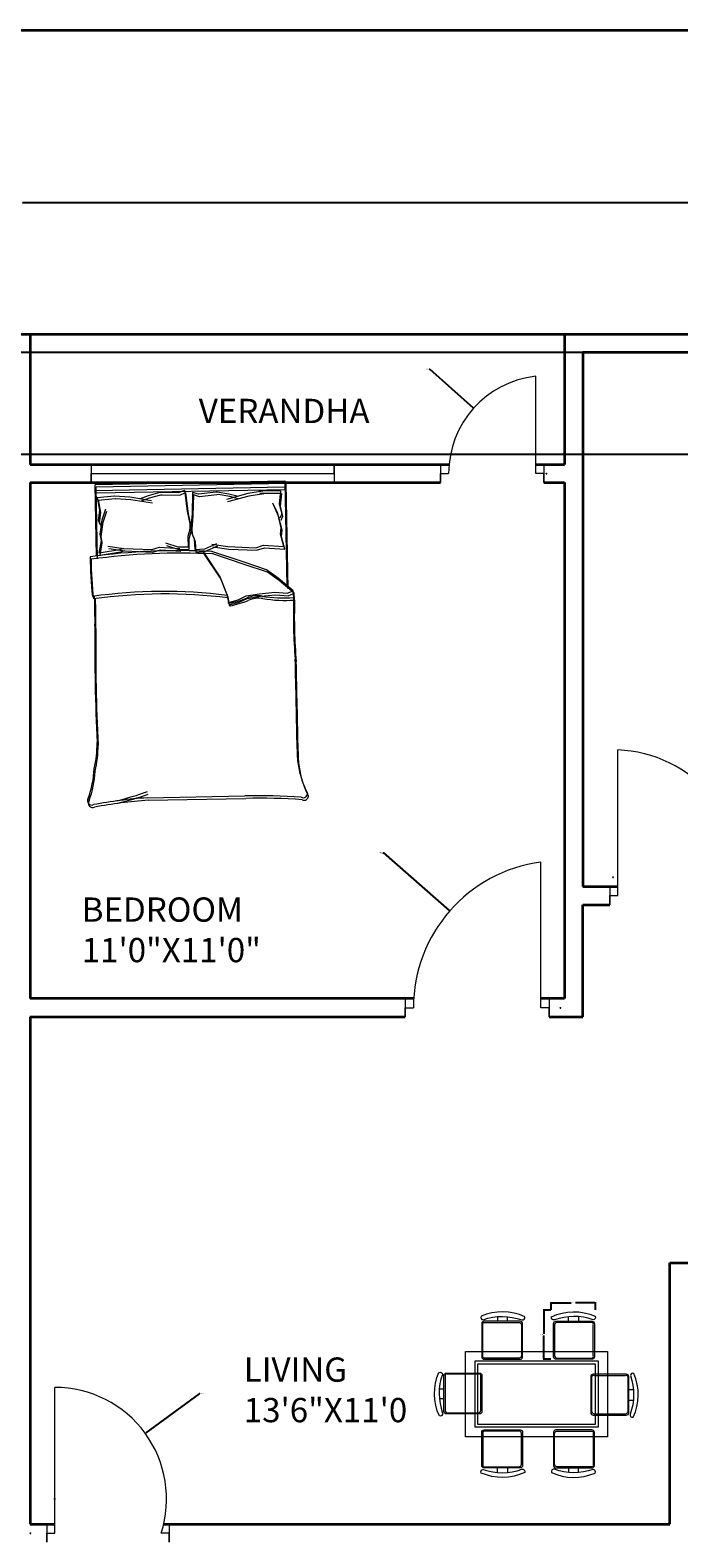
# Model space of a CAD drawing. Units: inches. Extents: x 1721 to 2510, y 1544 to 2360.
# Tile 9 of 10: x 2090 to 2250, y 1988 to 2360. Entities that reach past the tile are written whole.
import ezdxf

# ---------------------------------------------------------------- set-up
doc = ezdxf.new("R2010")
doc.units = ezdxf.units.IN
for name, color, linetype, lineweight in [('A-ANNO-DIMS', 2, 'Continuous', 18), ('A-ANNO-TTLB', 7, 'Continuous', 35), ('A-AREA-IDEN', 7, 'Continuous', 18), ('A-DOOR', 3, 'Continuous', 18), ('A-FURN', 8, 'Continuous', 13), ('A-GLAZ', 4, 'Continuous', 18), ('A-WALL', 7, 'Continuous', 35)]:
    doc.layers.add(name, color=color, linetype=linetype, lineweight=lineweight)
doc.styles.get("Standard").update_dxf_attribs({"font": 'arial.ttf'})
doc.dimstyles.get("Standard").update_dxf_attribs({"dimtxt": 0.18, "dimasz": 0.18, "dimexe": 0.18, "dimexo": 0.0625, "dimgap": 0.09, "dimtad": 0, "dimtih": 1, "dimtoh": 1, "dimdec": 4, "dimzin": 0, "dimdsep": 46, "dimtxsty": 'Standard', "dimcen": 0.09, "dimadec": 0, "dimazin": 0, "dimtfac": 1, "dimtdec": 4, "dimtofl": 0, "dimtmove": 0, "dimatfit": 3, "dimfxl": 1, "dimtolj": 1, "dimtzin": 0, "dimarcsym": 0})

# ---------------------------------------------------------------- blocks, each defined once
blk = doc.blocks.new('BED-DOUBLE')
for p, q in [((39.64, 78.43), (15.52, 78.72)), ((39.64, 78.43), (15.52, 78.72)), ((39.86, 77.8), (15.74, 78.09)), ((39.86, 77.8), (15.74, 78.09)), ((1.93, 30.11), (1.99, 28.4, 3.79)), ((1.93, 30.11), (1.99, 28.4, 3.79)), ((15.66, 30.21), (13.68, 29.32)), ((15.66, 30.21), (13.68, 29.32)), ((18.1, 30.79), (15.66, 30.21)), ((18.1, 30.79), (15.66, 30.21)), ((18.31, 30.16), (15.88, 29.58)), ((18.31, 30.16), (15.88, 29.58)), ((18.38, 28.81), (18.1, 30.79)), ((18.38, 28.81), (18.1, 30.79)), ((18.59, 28.18), (18.31, 30.16)), ((18.59, 28.18), (18.31, 30.16)), ((3.5, 28.99), (1.99, 28.4)), ((3.5, 28.99), (1.99, 28.4)), ((1.99, 28.4), (5.58, 25.17)), ((1.99, 28.4), (5.58, 25.17)), ((2.15, 29.48), (2.21, 27.77, 3.79)), ((2.15, 29.48), (2.21, 27.77, 3.79)), ((3.72, 28.36), (2.21, 27.77)), ((3.72, 28.36), (2.21, 27.77)), ((2.21, 27.77), (5.8, 24.54)), ((2.21, 27.77), (5.8, 24.54)), ((3.23, 1.19), (3.55, 27.27)), ((3.23, 1.19), (3.55, 27.27)), ((3.45, 0.56), (3.76, 26.64)), ((3.45, 0.56), (3.76, 26.64)), ((6.54, 28.65), (3.5, 28.99)), ((6.54, 28.65), (3.5, 28.99)), ((6.75, 28.02), (3.72, 28.36)), ((6.75, 28.02), (3.72, 28.36)), ((10.33, 28.91), (6.54, 28.65)), ((10.33, 28.91), (6.54, 28.65)), ((10.55, 28.28), (6.75, 28.02)), ((10.55, 28.28), (6.75, 28.02)), ((13.68, 29.32), (10.33, 28.91)), ((13.68, 29.32), (10.33, 28.91)), ((13.89, 28.69), (10.55, 28.28)), ((13.89, 28.69), (10.55, 28.28)), ((15.88, 29.58), (13.89, 28.69)), ((15.88, 29.58), (13.89, 28.69)), ((20, 24.39), (18.38, 28.81)), ((20, 24.39), (18.38, 28.81)), ((20.21, 23.76), (18.59, 28.18)), ((20.21, 23.76), (18.59, 28.18)), ((5.58, 25.17), (8.44, 23.01)), ((5.58, 25.17), (8.44, 23.01)), ((5.8, 24.54), (8.66, 22.38)), ((5.8, 24.54), (8.66, 22.38)), ((8.44, 23.01), (13.88, 20.98)), ((8.44, 23.01), (13.88, 20.98)), ((8.66, 22.38), (14.1, 20.35)), ((8.66, 22.38), (14.1, 20.35)), ((24.03, 17.98), (20, 24.39)), ((24.03, 17.98), (20, 24.39)), ((24.24, 17.35), (20.21, 23.76)), ((24.24, 17.35), (20.21, 23.76)), ((13.88, 20.98), (22.02, 18)), ((13.88, 20.98), (22.02, 18)), ((14.1, 20.35), (22.24, 17.37)), ((14.1, 20.35), (22.24, 17.37)), ((9.01, 16.97), (3.98, 17.42)), ((3.98, 17.42), (4.71, 14.34)), ((9.01, 16.97), (3.98, 17.42)), ((3.98, 17.42), (4.71, 14.34)), ((9.23, 16.34), (4.2, 16.8)), ((4.2, 16.8), (4.92, 13.71)), ((9.23, 16.34), (4.2, 16.8)), ((4.2, 16.8), (4.92, 13.71)), ((10.94, 17.49), (9.01, 16.97)), ((10.94, 17.49), (9.01, 16.97)), ((11.15, 16.86), (9.23, 16.34)), ((11.15, 16.86), (9.23, 16.34)), ((17.8, 16.99), (10.94, 17.49)), ((17.8, 16.99), (10.94, 17.49)), ((18.02, 16.36), (11.15, 16.86)), ((18.02, 16.36), (11.15, 16.86)), ((21.75, 16.29), (17.8, 16.99)), ((21.75, 16.29), (17.8, 16.99)), ((21.96, 15.66), (18.02, 16.36)), ((21.96, 15.66), (18.02, 16.36)), ((23.54, 17.35), (20.51, 16.13)), ((23.54, 17.35), (20.51, 16.13)), ((23.75, 16.73), (20.73, 15.5)), ((23.75, 16.73), (20.73, 15.5)), ((25.94, 17.48), (23.54, 17.35)), ((25.94, 17.48), (23.54, 17.35)), ((26.16, 16.85), (23.75, 16.73)), ((26.16, 16.85), (23.75, 16.73)), ((26.07, 14.85), (25.94, 17.48)), ((26.07, 14.85), (25.94, 17.48)), ((26.29, 14.22), (26.16, 16.85)), ((26.29, 14.22), (26.16, 16.85)), ((27.61, 14.21), (27.64, 16.84)), ((27.61, 14.21), (27.64, 16.84)), ((27.64, 16.84), (30.05, 16.81)), ((27.64, 16.84), (30.05, 16.81)), ((27.82, 13.58), (27.85, 16.21)), ((27.82, 13.58), (27.85, 16.21)), ((27.85, 16.21), (30.26, 16.18)), ((27.85, 16.21), (30.26, 16.18)), ((34.67, 16.66), (29.65, 17.12)), ((34.67, 16.66), (29.65, 17.12)), ((34.89, 16.03), (29.86, 16.49)), ((34.89, 16.03), (29.86, 16.49)), ((30.05, 16.81), (33.11, 15.7)), ((30.05, 16.81), (33.11, 15.7)), ((30.26, 16.18), (33.33, 15.07)), ((30.26, 16.18), (33.33, 15.07)), ((36.6, 17.19), (34.67, 16.66)), ((36.6, 17.19), (34.67, 16.66)), ((36.81, 16.56), (34.89, 16.03)), ((36.81, 16.56), (34.89, 16.03)), ((43.46, 16.68), (36.6, 17.19)), ((43.46, 16.68), (36.6, 17.19)), ((43.68, 16.05), (36.81, 16.56)), ((43.68, 16.05), (36.81, 16.56)), ((43.46, 16.68), (44.58, 16.98)), ((43.46, 16.68), (44.58, 16.98)), ((47.41, 15.98), (43.46, 16.68)), ((47.41, 15.98), (43.46, 16.68)), ((43.68, 16.05), (44.79, 16.35)), ((43.68, 16.05), (44.79, 16.35)), ((47.62, 15.35), (43.68, 16.05)), ((47.62, 15.35), (43.68, 16.05)), ((44.58, 16.98), (49.58, 17.63)), ((44.58, 16.98), (49.58, 17.63)), ((44.79, 16.35), (49.8, 17)), ((44.79, 16.35), (49.8, 17)), ((49.58, 17.63), (48.98, 14.52)), ((49.58, 17.63), (48.98, 14.52)), ((49.8, 17), (49.19, 13.89)), ((49.8, 17), (49.19, 13.89)), ((50.28, 18.38), (50.07, 0.63)), ((50.28, 18.38), (50.07, 0.63)), ((50.5, 17.75), (50.29, 0)), ((50.5, 17.75), (50.29, 0)), ((4.71, 14.34), (4.5, 12.77)), ((4.71, 14.34), (4.5, 12.77)), ((4.5, 12.77), (5.25, 9.26)), ((4.5, 12.77), (5.25, 9.26)), ((4.92, 13.71), (4.72, 12.14)), ((4.92, 13.71), (4.72, 12.14)), ((4.72, 12.14), (5.46, 8.63)), ((4.72, 12.14), (5.46, 8.63)), ((26.73, 13.04), (26.07, 14.85)), ((26.73, 13.04), (26.07, 14.85)), ((26.95, 12.41), (26.29, 14.22)), ((26.95, 12.41), (26.29, 14.22)), ((26.39, 8.62), (26.8, 11.77)), ((26.39, 8.62), (26.8, 11.77)), ((26.8, 11.77), (26.73, 13.04)), ((26.8, 11.77), (26.73, 13.04)), ((27.01, 11.14), (26.95, 12.41)), ((27.01, 11.14), (26.95, 12.41)), ((27, 11.1), (27.02, 12.38)), ((27, 11.1), (27.02, 12.38)), ((27.02, 12.38), (27.61, 14.21)), ((27.02, 12.38), (27.61, 14.21)), ((27.22, 10.47), (27.23, 11.75)), ((27.22, 10.47), (27.23, 11.75)), ((27.23, 11.75), (27.82, 13.58)), ((27.23, 11.75), (27.82, 13.58)), ((49.24, 12.96), (48.63, 9.42)), ((49.24, 12.96), (48.63, 9.42)), ((49.46, 12.33), (48.85, 8.79)), ((49.46, 12.33), (48.85, 8.79)), ((48.98, 14.52), (49.24, 12.96)), ((48.98, 14.52), (49.24, 12.96)), ((49.19, 13.89), (49.46, 12.33)), ((49.19, 13.89), (49.46, 12.33)), ((4.25, 9.35), (4.77, 10.37)), ((4.25, 9.35), (4.77, 10.37)), ((4.8, 6.82), (4.25, 9.35)), ((4.8, 6.82), (4.25, 9.35)), ((4.47, 8.72), (4.98, 9.74)), ((4.47, 8.72), (4.98, 9.74)), ((5.02, 6.19), (4.47, 8.72)), ((5.02, 6.19), (4.47, 8.72)), ((5.25, 9.26), (6.37, 6.62)), ((5.25, 9.26), (6.37, 6.62)), ((5.46, 8.63), (6.59, 5.99)), ((5.46, 8.63), (6.59, 5.99)), ((26.09, 3.36), (26.39, 8.62)), ((26.09, 3.36), (26.39, 8.62)), ((26.3, 2.73), (26.61, 7.99)), ((26.3, 2.73), (26.61, 7.99)), ((26.61, 7.99), (27.01, 11.14)), ((26.61, 7.99), (27.01, 11.14)), ((27.53, 7.98), (27, 11.1)), ((27.53, 7.98), (27, 11.1)), ((27.75, 7.35), (27.22, 10.47)), ((27.75, 7.35), (27.22, 10.47)), ((28.04, 2.73), (27.53, 7.98)), ((28.04, 2.73), (27.53, 7.98)), ((48.63, 9.42), (47.61, 6.74)), ((48.63, 9.42), (47.61, 6.74)), ((48.85, 8.79), (47.82, 6.11)), ((48.85, 8.79), (47.82, 6.11)), ((49.63, 9.55), (49.07, 10.55)), ((49.63, 9.55), (49.07, 10.55)), ((49.17, 7.01), (49.63, 9.55)), ((49.17, 7.01), (49.63, 9.55)), ((49.84, 8.92), (49.29, 9.92)), ((49.84, 8.92), (49.29, 9.92)), ((49.39, 6.38), (49.84, 8.92)), ((49.39, 6.38), (49.84, 8.92)), ((4.39, 3.68), (4.8, 6.82)), ((4.39, 3.68), (4.8, 6.82)), ((4.61, 3.05), (5.02, 6.19)), ((4.61, 3.05), (5.02, 6.19)), ((8.71, 3.62), (12.44, 4.09)), ((8.71, 3.62), (12.44, 4.09)), ((12.44, 4.09), (17.76, 5.35)), ((12.44, 4.09), (17.76, 5.35)), ((12.65, 3.46), (17.98, 4.72)), ((12.65, 3.46), (17.98, 4.72)), ((15.1, 4.65), (17.12, 4.04)), ((15.1, 4.65), (17.12, 4.04)), ((15.32, 4.02), (17.34, 3.41)), ((15.32, 4.02), (17.34, 3.41)), ((17.12, 4.04), (19.98, 3.48)), ((17.12, 4.04), (19.98, 3.48)), ((20.3, 3.49), (24.64, 3.85)), ((20.3, 3.49), (24.64, 3.85)), ((24.64, 3.85), (26.09, 3.36)), ((24.64, 3.85), (26.09, 3.36)), ((28.25, 2.1), (27.75, 7.35)), ((28.25, 2.1), (27.75, 7.35)), ((36.97, 3.75), (34.13, 3.08)), ((36.97, 3.75), (34.13, 3.08)), ((41.65, 3.98), (36.28, 5.04)), ((41.65, 3.98), (36.28, 5.04)), ((41.87, 3.35), (36.49, 4.41)), ((41.87, 3.35), (36.49, 4.41)), ((38.96, 4.44), (36.97, 3.75)), ((38.96, 4.44), (36.97, 3.75)), ((39.18, 3.81), (37.19, 3.12)), ((39.18, 3.81), (37.19, 3.12)), ((45.39, 3.65), (41.65, 3.98)), ((45.39, 3.65), (41.65, 3.98)), ((49.7, 3.91), (45.5, 3.63)), ((49.7, 3.91), (45.5, 3.63)), ((49.7, 3.88), (49.17, 7.01)), ((49.7, 3.88), (49.17, 7.01)), ((49.92, 3.25), (49.39, 6.38)), ((49.92, 3.25), (49.39, 6.38)), ((50.07, 0.63), (3.23, 1.19)), ((50.07, 0.63), (3.23, 1.19)), ((50.09, 2.13), (3.25, 2.69)), ((50.09, 2.13), (3.25, 2.69)), ((50.29, 0), (3.45, 0.56)), ((50.29, 0), (3.45, 0.56)), ((50.31, 1.5), (3.47, 2.06)), ((50.31, 1.5), (3.47, 2.06)), ((4.39, 3.68), (9.69, 3.52)), ((4.39, 3.68), (9.69, 3.52)), ((4.61, 3.05), (9.9, 2.89)), ((4.61, 3.05), (9.9, 2.89)), ((9.69, 3.52), (8.71, 3.62)), ((9.69, 3.52), (8.71, 3.62)), ((8.92, 2.99), (12.65, 3.46)), ((8.92, 2.99), (12.65, 3.46)), ((9.9, 2.89), (8.92, 2.99)), ((9.9, 2.89), (8.92, 2.99)), ((17.34, 3.41), (20.2, 2.85)), ((17.34, 3.41), (20.2, 2.85)), ((19.98, 3.48), (20.3, 3.49)), ((19.98, 3.48), (20.3, 3.49)), ((20.2, 2.85), (20.52, 2.86)), ((20.2, 2.85), (20.52, 2.86)), ((20.52, 2.86), (24.86, 3.22)), ((20.52, 2.86), (24.86, 3.22)), ((24.86, 3.22), (26.3, 2.73)), ((24.86, 3.22), (26.3, 2.73)), ((29.46, 3.28), (28.04, 2.73)), ((29.46, 3.28), (28.04, 2.73)), ((29.68, 2.65), (28.25, 2.1)), ((29.68, 2.65), (28.25, 2.1)), ((33.81, 3.08), (29.46, 3.28)), ((33.81, 3.08), (29.46, 3.28)), ((34.03, 2.45), (29.68, 2.65)), ((34.03, 2.45), (29.68, 2.65)), ((34.13, 3.08), (33.81, 3.08)), ((34.13, 3.08), (33.81, 3.08)), ((34.35, 2.45), (34.03, 2.45)), ((34.35, 2.45), (34.03, 2.45)), ((37.19, 3.12), (34.35, 2.45)), ((37.19, 3.12), (34.35, 2.45)), ((45.61, 3.02), (41.87, 3.35)), ((45.61, 3.02), (41.87, 3.35)), ((45.5, 3.63), (45.39, 3.65)), ((45.5, 3.63), (45.39, 3.65)), ((45.71, 3), (45.61, 3.02)), ((45.71, 3), (45.61, 3.02)), ((49.91, 3.28), (45.71, 3)), ((49.91, 3.28), (45.71, 3))]:
    blk.add_line(p, q)
for centre, radius, start, end in [((1.08, 78.52), 1.08, 61.9736, 175.3348), ((1.08, 78.52), 1.08, 61.9736, 175.3348), ((-20.36, 68.78), 22.61, 356.7862, 25.7829), ((-20.36, 68.78), 22.61, 356.7862, 25.7829), ((1.29, 77.89), 1.08, 61.9736, 175.3348), ((1.29, 77.89), 1.08, 61.9736, 175.3348), ((15.63, 209.12), 130.4, 263.8146, 269.9499), ((15.63, 209.12), 130.4, 263.8146, 269.9499), ((15.85, 208.49), 130.4, 263.8146, 269.9499), ((15.85, 208.49), 130.4, 263.8146, 269.9499), ((70.08, -22.85), 104.34, 102.698, 107.0202), ((70.08, -22.85), 104.34, 102.698, 107.0202), ((34.83, 197.67), 119.34, 272.3106, 278.7239), ((34.83, 197.67), 119.34, 272.3106, 278.7239), ((70.29, -23.48), 104.34, 102.698, 107.0202), ((70.29, -23.48), 104.34, 102.698, 107.0202), ((35.05, 197.04), 119.34, 272.3106, 278.7239), ((35.05, 197.04), 119.34, 272.3106, 278.7239), ((53.35, 78.73), 1.07, 325.4884, 112.793), ((53.35, 78.73), 1.07, 325.4884, 112.793), ((53.56, 78.1), 1.07, 325.4884, 112.793), ((53.56, 78.1), 1.07, 325.4884, 112.793), ((-20.14, 68.15), 22.61, 356.7862, 25.7829), ((-20.14, 68.15), 22.61, 356.7862, 25.7829), ((75.53, 69.21), 23.09, 157.2899, 175.9668), ((75.53, 69.21), 23.09, 157.2899, 175.9668), ((75.75, 68.58), 23.09, 157.2899, 175.9668), ((75.75, 68.58), 23.09, 157.2899, 175.9668), ((80.6, 63.5), 29.05, 165.3797, 178.2261), ((80.6, 63.5), 29.05, 165.3797, 178.2261), ((4473.12, 14.21), 4471.22, 179.317, 179.60172), ((4473.12, 14.21), 4471.22, 179.317, 179.60172), ((80.81, 62.87), 29.05, 165.3797, 178.2261), ((80.81, 62.87), 29.05, 165.3797, 178.2261), ((4473.34, 13.58), 4471.22, 179.317, 179.60172), ((4473.34, 13.58), 4471.22, 179.317, 179.60172), ((-421.08, 55.88), 472.73, 357.5425, 1.0334), ((-421.08, 55.88), 472.73, 357.5425, 1.0334), ((-420.87, 55.25), 472.73, 357.5425, 1.0334), ((-420.87, 55.25), 472.73, 357.5425, 1.0334), ((-124.73, 38.32), 126.93, 356.294, 3.1513), ((-124.73, 38.32), 126.93, 356.294, 3.1513), ((-124.51, 37.69), 126.93, 356.294, 3.1513), ((-124.51, 37.69), 126.93, 356.294, 3.1513), ((217.81, 29.18), 166.73, 177.791, 180.323), ((217.81, 29.18), 166.73, 177.791, 180.323), ((218.03, 28.55), 166.73, 177.791, 180.323), ((218.03, 28.55), 166.73, 177.791, 180.323), ((3.1, -5.33), 35.46, 79.1911, 91.8805), ((3.1, -5.33), 35.46, 79.1911, 91.8805), ((11.02, 35.47), 6.1, 257.9756, 293.0532), ((11.02, 35.47), 6.1, 257.9756, 293.0532), ((22.96, 2.41), 29.06, 99.9765, 109.1954), ((22.96, 2.41), 29.06, 99.9765, 109.1954), ((23.18, 1.78), 29.06, 99.9765, 109.1954), ((23.18, 1.78), 29.06, 99.9765, 109.1954), ((17.93, 30.85), 0.181, 339.5612, 90.4525), ((17.93, 30.85), 0.181, 339.5612, 90.4525), ((18.15, 30.22), 0.181, 339.5612, 90.4525), ((18.15, 30.22), 0.181, 339.5612, 90.4525), ((3.31, -5.96), 35.46, 79.1911, 91.8805), ((3.31, -5.96), 35.46, 79.1911, 91.8805), ((11.23, 34.84), 6.1, 257.9756, 293.0532), ((11.23, 34.84), 6.1, 257.9756, 293.0532), ((37.91, 154), 126.46, 261.0993, 276.2154), ((37.91, 154), 126.46, 261.0993, 276.2154), ((38.12, 153.37), 126.46, 261.0993, 276.2154), ((38.12, 153.37), 126.46, 261.0993, 276.2154), ((-29.75, 21.28), 81.65, 358.0366, 4.9188), ((-29.75, 21.28), 81.65, 358.0366, 4.9188), ((-29.53, 20.65), 81.65, 358.0366, 4.9188), ((-29.53, 20.65), 81.65, 358.0366, 4.9188), ((34.68, 179.26), 161.69, 265.4014, 276.097), ((34.68, 179.26), 161.69, 265.4014, 276.097), ((34.89, 178.63), 161.69, 265.4014, 276.097), ((34.89, 178.63), 161.69, 265.4014, 276.097)]:
    blk.add_arc(centre, radius, start, end)
blk = doc.blocks.new('WIN-60IN-A')
for p, q in [((4.5, 60), (0, 60)), ((2.25, 0), (2.25, 60)), ((2.25, 60), (4.5, 60)), ((4.5, 0), (0, 0)), ((0, 0), (2.25, 0))]:
    blk.add_line(p, q)
blk = doc.blocks.new('TABLE-DINING-RECT')
for points in [[(0, 21.04), (35.07, 21.04), (35.07, 0), (0, 0)], [(2.34, 18.71), (32.73, 18.71), (32.73, 2.34), (2.34, 2.34)], [(3.04, 18), (32.03, 18), (32.03, 3.04), (3.04, 3.04)]]:
    blk.add_lwpolyline(points, close=True)
blk = doc.blocks.new('CHAIR-DINING-D')
for points in [[(0.75, 9.71, -0.578392), (0.03, 10.5, -0.214524), (10.81, 10.65, -0.552014), (10.31, 9.78, 0.175809), (0.75, 9.71)], [(10.03, 9.4, -0.414214), (10.65, 8.78), (10.65, 0.62, -0.414214), (10.03, 0), (1.16, 0, -0.414214), (0.54, 0.62), (0.54, 8.78, -0.414214), (1.16, 9.4), (10.03, 9.4)], [(4.27, 9.4), (4.27, 10.52, 0.064759)]]:
    blk.add_lwpolyline(points, format="xyb")
blk.add_lwpolyline([(10.02, 9.12), (1.44, 9.12, 0.414214), (0.82, 8.5), (0.82, 0.9, 0.414214), (1.44, 0.28), (10.02, 0.28, 0.512069), (10.37, 0.9), (10.37, 8.5, 0.512069)], format="xyb", close=True)
blk.add_lwpolyline([(6.76, 10.54), (6.76, 9.4)])
blk = doc.blocks.new('CHAIR-DINING-E')
for points in [[(9.4, 10.03, 0.414214), (8.77, 10.65), (0.62, 10.65, 0.414214), (0, 10.03), (0, 1.16, 0.414214), (0.62, 0.54), (8.77, 0.54, 0.414214), (9.4, 1.16), (9.4, 10.03)], [(9.78, 10.31, -0.175809), (9.71, 0.75, 0.578392), (10.5, 0.03, 0.214524), (10.65, 10.81, 0.552014), (9.78, 10.31, -0.065079)], [(9.4, 4.27), (10.52, 4.27, -0.064759)]]:
    blk.add_lwpolyline(points, format="xyb")
blk.add_lwpolyline([(9.12, 10.02), (9.12, 1.44, -0.414214), (8.5, 0.82), (0.9, 0.82, -0.414214), (0.28, 1.44), (0.28, 10.02, -0.512069), (0.9, 10.37), (8.5, 10.37, -0.512069)], format="xyb", close=True)
blk.add_lwpolyline([(10.54, 6.76), (9.4, 6.76)])
blk = doc.blocks.new('*D36')
at = {"layer": 'A-ANNO-DIMS', "color": 0, "lineweight": -2, "transparency": 16777216}
for p, q in [((2218.14, 2043.98), (2216.2, 2043.98)), ((2216.38, 2043.8), (2216.38, 2038.09)), ((2216.38, 2032.01), (2216.38, 2037.72)), ((2218.14, 2031.83), (2216.2, 2031.83))]:
    blk.add_line(p, q, dxfattribs=at)
at = {"layer": 'A-ANNO-DIMS', "color": 0, "transparency": 16777216}
for points in [[(2216.35, 2043.8), (2216.41, 2043.8), (2216.38, 2043.98)], [(2216.35, 2032.01), (2216.41, 2032.01), (2216.38, 2031.83)]]:
    blk.add_solid(points, dxfattribs=at)
at = {"layer": 'Defpoints', "color": 0, "transparency": 16777216}
for p in [(2216.38, 2043.98), (2218.2, 2043.98), (2218.2, 2031.83)]:
    blk.add_point(p, dxfattribs=at)
at = {"layer": 'A-ANNO-DIMS', "color": 0, "transparency": 16777216, "insert": (2216.38, 2037.9), "char_height": 0.18, "attachment_point": 5}
blk.add_mtext('\\A1;CHAIR D 12 TYP.', dxfattribs=at)
blk = doc.blocks.new('*D37')
at = {"layer": 'A-ANNO-DIMS', "color": 0, "lineweight": -2, "transparency": 16777216}
for p, q in [((2218.2, 2044.04), (2218.2, 2045.98)), ((2218.38, 2045.8), (2223.16, 2045.8)), ((2228.97, 2045.8), (2224.2, 2045.8)), ((2229.15, 2044.04), (2229.15, 2045.98))]:
    blk.add_line(p, q, dxfattribs=at)
at = {"layer": 'A-ANNO-DIMS', "color": 0, "transparency": 16777216}
for points in [[(2218.38, 2045.83), (2218.38, 2045.77), (2218.2, 2045.8)], [(2228.97, 2045.83), (2228.97, 2045.77), (2229.15, 2045.8)]]:
    blk.add_solid(points, dxfattribs=at)
at = {"layer": 'Defpoints', "color": 0, "transparency": 16777216}
for p in [(2229.15, 2045.8), (2218.2, 2043.98), (2229.15, 2043.98)]:
    blk.add_point(p, dxfattribs=at)
at = {"layer": 'A-ANNO-DIMS', "color": 0, "transparency": 16777216, "insert": (2223.68, 2045.8), "char_height": 0.18, "attachment_point": 5}
blk.add_mtext('\\A1;11 TYP.', dxfattribs=at)
blk = doc.blocks.new('*D40')
at = {"layer": 'A-ANNO-DIMS', "color": 0, "lineweight": -2, "transparency": 16777216}
for p, q in [((1798, 2285.19), (1798, 2317.71)), ((1798.18, 2317.53), (2086.86, 2317.53)), ((2376.32, 2317.53), (2087.65, 2317.53)), ((2376.5, 2285.19), (2376.5, 2317.71))]:
    blk.add_line(p, q, dxfattribs=at)
at = {"layer": 'A-ANNO-DIMS', "color": 0, "transparency": 16777216}
for points in [[(1798.18, 2317.56), (1798.18, 2317.5), (1798, 2317.53)], [(2376.32, 2317.56), (2376.32, 2317.5), (2376.5, 2317.53)]]:
    blk.add_solid(points, dxfattribs=at)
at = {"layer": 'Defpoints', "color": 0, "transparency": 16777216}
for p in [(2376.5, 2317.53), (1798, 2285.13), (2376.5, 2285.13)]:
    blk.add_point(p, dxfattribs=at)
at = {"layer": 'A-ANNO-DIMS', "color": 0, "transparency": 16777216, "insert": (2087.25, 2317.53), "char_height": 0.18, "attachment_point": 5}
blk.add_mtext('\\A1;578.5', dxfattribs=at)
blk = doc.blocks.new('*D57')
at = {"layer": 'A-ANNO-DIMS', "color": 0, "lineweight": -2, "transparency": 16777216}
for p, q in [((1802.56, 2280.63), (2409.08, 2280.63)), ((2408.9, 2280.45), (2408.9, 2268.22)), ((2408.9, 2255.63), (2408.9, 2267.86)), ((1802.56, 2255.45), (2409.08, 2255.45))]:
    blk.add_line(p, q, dxfattribs=at)
at = {"layer": 'A-ANNO-DIMS', "color": 0, "transparency": 16777216}
for points in [[(2408.87, 2280.45), (2408.93, 2280.45), (2408.9, 2280.63)], [(2408.87, 2255.63), (2408.93, 2255.63), (2408.9, 2255.45)]]:
    blk.add_solid(points, dxfattribs=at)
at = {"layer": 'Defpoints', "color": 0, "transparency": 16777216}
for p in [(1802.5, 2280.63), (1802.5, 2255.45), (2408.9, 2255.45)]:
    blk.add_point(p, dxfattribs=at)
at = {"layer": 'A-ANNO-DIMS', "color": 0, "transparency": 16777216, "insert": (2408.9, 2268.04), "char_height": 0.18, "attachment_point": 5}
blk.add_mtext('\\A1;25.18', dxfattribs=at)
blk = doc.blocks.new('*D68')
at = {"layer": 'A-ANNO-DIMS', "color": 0, "lineweight": -2, "transparency": 16777216}
for p, q in [((2040.83, 2024.64), (2041.01, 2024.64)), ((2041.01, 2024.64), (2059.08, 2011.34)), ((2089.5, 1988.88), (2089.68, 1988.88)), ((2089.59, 1988.79), (2089.59, 1988.97))]:
    blk.add_line(p, q, dxfattribs=at)
at = {"layer": 'A-ANNO-DIMS', "color": 0, "transparency": 16777216}
blk.add_solid([(2059.1, 2011.36), (2059.06, 2011.31), (2059.23, 2011.23)], dxfattribs=at)
at = {"layer": 'Defpoints', "color": 0, "transparency": 16777216}
for p in [(2059.23, 2011.23), (2089.59, 1988.88)]:
    blk.add_point(p, dxfattribs=at)
at = {"layer": 'A-ANNO-DIMS', "color": 0, "transparency": 16777216, "insert": (2040.42, 2024.64), "char_height": 0.18, "attachment_point": 5}
blk.add_mtext('\\A1;R37.7', dxfattribs=at)
blk = doc.blocks.new('*D72')
at = {"layer": 'A-ANNO-DIMS', "color": 0, "lineweight": -2, "transparency": 16777216}
for p, q in [((2176.59, 2156.96), (2176.77, 2156.96)), ((2176.77, 2156.96), (2193.03, 2142.73)), ((2220.42, 2118.69), (2220.6, 2118.69)), ((2220.51, 2118.6), (2220.51, 2118.78))]:
    blk.add_line(p, q, dxfattribs=at)
at = {"layer": 'A-ANNO-DIMS', "color": 0, "transparency": 16777216}
blk.add_solid([(2193.05, 2142.75), (2193.01, 2142.7), (2193.17, 2142.61)], dxfattribs=at)
at = {"layer": 'Defpoints', "color": 0, "transparency": 16777216}
for p in [(2193.17, 2142.61), (2220.51, 2118.69)]:
    blk.add_point(p, dxfattribs=at)
at = {"layer": 'A-ANNO-DIMS', "color": 0, "transparency": 16777216, "insert": (2176.11, 2156.96), "char_height": 0.18, "attachment_point": 5}
blk.add_mtext('\\A1;R36.32', dxfattribs=at)
blk = doc.blocks.new('*D76')
at = {"layer": 'A-ANNO-DIMS', "color": 0, "lineweight": -2, "transparency": 16777216}
for p, q in [((2272.21, 2183.16), (2257.85, 2171.2)), ((2272.39, 2183.16), (2272.21, 2183.16)), ((2233.46, 2150.95), (2233.64, 2150.95)), ((2233.55, 2150.86), (2233.55, 2151.04))]:
    blk.add_line(p, q, dxfattribs=at)
at = {"layer": 'A-ANNO-DIMS', "color": 0, "transparency": 16777216}
blk.add_solid([(2257.83, 2171.22), (2257.87, 2171.17), (2257.71, 2171.08)], dxfattribs=at)
at = {"layer": 'Defpoints', "color": 0, "transparency": 16777216}
for p in [(2257.71, 2171.08), (2233.55, 2150.95)]:
    blk.add_point(p, dxfattribs=at)
at = {"layer": 'A-ANNO-DIMS', "color": 0, "transparency": 16777216, "insert": (2272.93, 2183.16), "char_height": 0.18, "attachment_point": 5}
blk.add_mtext('\\A1;R31.446', dxfattribs=at)
blk = doc.blocks.new('*D82')
at = {"layer": 'A-ANNO-DIMS', "color": 0, "lineweight": -2, "transparency": 16777216}
for p, q in [((2131.27, 2023.3), (2118.05, 2013.66)), ((2131.45, 2023.3), (2131.27, 2023.3)), ((2095.54, 1997.31), (2095.72, 1997.31)), ((2095.63, 1997.22), (2095.63, 1997.4))]:
    blk.add_line(p, q, dxfattribs=at)
at = {"layer": 'A-ANNO-DIMS', "color": 0, "transparency": 16777216}
blk.add_solid([(2118.03, 2013.68), (2118.07, 2013.63), (2117.91, 2013.55)], dxfattribs=at)
at = {"layer": 'Defpoints', "color": 0, "transparency": 16777216}
for p in [(2117.91, 2013.55), (2095.63, 1997.31)]:
    blk.add_point(p, dxfattribs=at)
at = {"layer": 'A-ANNO-DIMS', "color": 0, "transparency": 16777216, "insert": (2131.93, 2023.3), "char_height": 0.18, "attachment_point": 5}
blk.add_mtext('\\A1;R27.57', dxfattribs=at)
blk = doc.blocks.new('*D84')
at = {"layer": 'A-ANNO-DIMS', "color": 0, "lineweight": -2, "transparency": 16777216}
for p, q in [((2188.09, 2276.48), (2188.27, 2276.48)), ((2188.27, 2276.48), (2198.92, 2266.93)), ((2216.94, 2250.69), (2217.12, 2250.69)), ((2217.03, 2250.6), (2217.03, 2250.78))]:
    blk.add_line(p, q, dxfattribs=at)
at = {"layer": 'A-ANNO-DIMS', "color": 0, "transparency": 16777216}
blk.add_solid([(2198.94, 2266.95), (2198.9, 2266.91), (2199.06, 2266.81)], dxfattribs=at)
at = {"layer": 'Defpoints', "color": 0, "transparency": 16777216}
for p in [(2199.06, 2266.81), (2217.03, 2250.69)]:
    blk.add_point(p, dxfattribs=at)
at = {"layer": 'A-ANNO-DIMS', "color": 0, "transparency": 16777216, "insert": (2187.54, 2276.48), "char_height": 0.18, "attachment_point": 5}
blk.add_mtext('\\A1;R24.143', dxfattribs=at)

msp = doc.modelspace()

# ---------------------------------------------------------------- linework, layer by layer
at = {"layer": 'A-ANNO-TTLB'}
msp.add_lwpolyline([(1721.1268, 2360.2177), (2509.707, 2360.2177), (2509.707, 1544.3037), (1721.1268, 1544.3037)], close=True, dxfattribs=at)
at = {"layer": 'A-DOOR'}
for p, q in [((2214.4091, 2250.6915), (2214.4091, 2274.6915)), ((2190.8892, 2252.9415), (2190.8892, 2248.4415)), ((2190.8892, 2248.4415), (2190.8892, 2250.6915)), ((2190.8892, 2250.6915), (2192.8892, 2250.6915)), ((2216.4091, 2250.6915), (2214.4091, 2250.6915)), ((2216.4091, 2252.9415), (2216.4091, 2248.4415)), ((2216.4091, 2248.4415), (2216.4091, 2250.6915)), ((2234.6695, 2146.3798), (2234.6695, 2182.3798)), ((2215.6811, 2118.6915), (2215.6811, 2154.6915)), ((2232.6695, 2148.6298), (2232.6695, 2144.1298)), ((2232.6695, 2144.1298), (2232.6695, 2146.3798)), ((2232.6695, 2146.3798), (2234.6695, 2146.3798)), ((2182.1841, 2120.9415), (2182.1841, 2116.4415)), ((2217.6811, 2120.9415), (2217.6811, 2116.4415)), ((2182.1841, 2116.4415), (2182.1841, 2118.6915)), ((2182.1841, 2118.6915), (2184.1841, 2118.6915)), ((2217.6811, 2118.6915), (2215.6811, 2118.6915)), ((2217.6811, 2116.4415), (2217.6811, 2118.6915)), ((2095.6307, 1988.8798), (2095.6307, 2024.8798)), ((2093.6307, 1991.1298), (2093.6307, 1986.6298)), ((2123.8777, 1991.1298), (2123.8777, 1986.6298)), ((2093.6307, 1986.6298), (2093.6307, 1988.8798)), ((2093.6307, 1988.8798), (2095.6307, 1988.8798)), ((2123.8777, 1988.8798), (2121.8777, 1988.8798)), ((2123.8777, 1986.6298), (2123.8777, 1988.8798))]:
    msp.add_line(p, q, dxfattribs=at)
for centre, radius, start, end in [((2217.0321, 2250.6915), 24.1429, 96.237086, 180), ((2233.549, 2150.9538), 31.446, 351.636388, 87.958091), ((2220.506, 2118.6915), 36.3219, 97.633615, 180), ((2095.6307, 1997.3117), 27.5681, 342.190239, 90)]:
    msp.add_arc(centre, radius, start, end, dxfattribs=at)
at = {"layer": 'A-FURN'}
for points in [[(2201.4014, 2041.611, -0.17580919), (2210.9543, 2041.5387, 0.57839206), (2211.678, 2042.3345, 0.21452438), (2200.8948, 2042.4791, 0.55201397), (2201.4014, 2041.611, -0.06507904)], [(2207.4339, 2041.2276), (2207.4339, 2042.3492, -0.06475861)], [(2210.549, 2041.2276), (2201.6804, 2041.2276, 0.41421356), (2201.06, 2040.6072), (2201.06, 2032.4527, 0.41421356), (2201.6804, 2031.8323), (2210.549, 2031.8323, 0.41421356), (2211.1694, 2032.4527), (2211.1694, 2040.6072, 0.41421356), (2210.549, 2041.2276)], [(2191.4073, 2018.5424, -0.57839206), (2190.6115, 2017.8187, -0.21452438), (2190.4669, 2028.6018, -0.55201397), (2191.335, 2028.0952, 0.17580937), (2191.4073, 2018.5424)], [(2191.7184, 2027.8162, -0.41421356), (2192.3388, 2028.4366), (2200.4933, 2028.4366, -0.41421356), (2201.1137, 2027.8162), (2201.1137, 2018.9477, -0.41421356), (2200.4933, 2018.3272), (2192.3388, 2018.3272, -0.41421356), (2191.7184, 2018.9477), (2191.7184, 2027.8162)], [(2191.7184, 2022.0627), (2190.5968, 2022.0627, 0.06475861)], [(2210.549, 2004.9791), (2201.6804, 2004.9791, -0.41421356), (2201.06, 2005.5996), (2201.06, 2013.754, -0.41421356), (2201.6804, 2014.3745), (2210.549, 2014.3745, -0.41421356), (2211.1694, 2013.754), (2211.1694, 2005.5996, -0.41421356), (2210.549, 2004.9791)], [(2228.2703, 2004.9791, 0.41421356), (2228.8908, 2005.5996), (2228.8908, 2013.754, 0.41421356), (2228.2703, 2014.3745), (2219.4018, 2014.3745, 0.41421356), (2218.7814, 2013.754), (2218.7814, 2005.5996, 0.41421356), (2219.4018, 2004.9791), (2228.2703, 2004.9791)], [(2210.9543, 2004.668, -0.57839206), (2211.678, 2003.8723, -0.21452438), (2200.8948, 2003.7276, -0.55201397), (2201.4014, 2004.5957, 0.17580929), (2210.9543, 2004.668)], [(2207.4339, 2004.9791), (2207.4339, 2003.8575, 0.06475861)], [(2228.5494, 2004.5957, -0.17580928), (2218.9965, 2004.668, 0.57839206), (2218.2728, 2003.8723, 0.21452438), (2229.056, 2003.7276, 0.55201397), (2228.5494, 2004.5957, -0.06507904)], [(2222.5169, 2004.9791), (2222.5169, 2003.8575, -0.06475861)]]:
    msp.add_lwpolyline(points, format="xyb", dxfattribs=at)
for points in [[(2204.9515, 2042.3696), (2204.9515, 2041.2276)], [(2190.5764, 2024.5452), (2191.7184, 2024.5452)], [(2204.9515, 2003.8371), (2204.9515, 2004.9791)], [(2224.9993, 2003.8371), (2224.9993, 2004.9791)]]:
    msp.add_lwpolyline(points, dxfattribs=at)
for points in [[(2201.6842, 2040.9481), (2210.2695, 2040.9481, -0.41421356), (2210.8899, 2040.3277), (2210.8899, 2032.7322, -0.41421356), (2210.2695, 2032.1118), (2201.6842, 2032.1118, -0.51206948), (2201.3395, 2032.7322), (2201.3395, 2040.3277, -0.51206948)], [(2191.9979, 2027.8124), (2191.9979, 2019.2272, 0.41421356), (2192.6183, 2018.6067), (2200.2138, 2018.6067, 0.41421356), (2200.8342, 2019.2272), (2200.8342, 2027.8124, 0.51206948), (2200.2138, 2028.1571), (2192.6183, 2028.1571, 0.51206948)], [(2201.6842, 2005.2586), (2210.2695, 2005.2586, 0.41421356), (2210.8899, 2005.8791), (2210.8899, 2013.4745, 0.41421356), (2210.2695, 2014.0949), (2201.6842, 2014.0949, 0.51206948), (2201.3395, 2013.4745), (2201.3395, 2005.8791, 0.51206948)], [(2228.2666, 2005.2586), (2219.6813, 2005.2586, -0.41421356), (2219.0609, 2005.8791), (2219.0609, 2013.4745, -0.41421356), (2219.6813, 2014.0949), (2228.2666, 2014.0949, -0.51206948), (2228.6113, 2013.4745), (2228.6113, 2005.8791, -0.51206948)]]:
    msp.add_lwpolyline(points, format="xyb", close=True, dxfattribs=at)
at = {"layer": 'A-WALL'}
for p, q in [((1953.0024, 2285.1298), (2221.5024, 2285.1298)), ((2085.0024, 2285.1298), (2089.5024, 2285.1298)), ((2089.5024, 2285.1298), (2089.5024, 2252.9415)), ((2221.5024, 2285.1298), (2221.5024, 2252.9415)), ((2221.5024, 2285.1298), (2376.5024, 2285.1298)), ((2226.0024, 2280.6298), (2226.0024, 2148.6298)), ((2226.0024, 2280.6298), (2372.0024, 2280.6298)), ((2089.5024, 2252.9415), (2192.9943, 2252.9415)), ((2214.4091, 2252.9415), (2221.5024, 2252.9415)), ((2089.5024, 2248.4415), (2089.5024, 2120.9415)), ((2089.5024, 2248.4415), (2190.8892, 2248.4415)), ((2216.4091, 2248.4415), (2221.5024, 2248.4415)), ((2221.5024, 2248.4415), (2221.5024, 2120.9415)), ((2221.5024, 2248.4415), (2221.5024, 2144.1298)), ((2226.0024, 2148.6298), (2234.6695, 2148.6298)), ((2226.0024, 2116.4415), (2226.0024, 2144.1298)), ((2226.0024, 2144.1298), (2232.6695, 2144.1298)), ((2184.2539, 2120.9415), (2089.5024, 2120.9415)), ((2221.5024, 2120.9415), (2215.6811, 2120.9415)), ((2089.5024, 2116.4415), (2089.5024, 1991.1298)), ((2089.5024, 2116.4415), (2182.1841, 2116.4415)), ((2217.6811, 2116.4415), (2226.0024, 2116.4415)), ((2247.5024, 2055.6298), (2255.717, 2055.6298)), ((2247.5024, 1991.1298), (2247.5024, 2055.6298)), ((2089.5024, 1991.1298), (2095.6307, 1991.1298)), ((2122.4967, 1991.1298), (2247.5024, 1991.1298))]:
    msp.add_line(p, q, dxfattribs=at)

# ---------------------------------------------------------------- block references
at = {"layer": 'A-FURN', "rotation": 181.7686830003587}
msp.add_blockref('BED-DOUBLE', (2155.8394, 2249.5507), dxfattribs=at)
at = {"layer": 'A-FURN'}
for name, p in [('CHAIR-DINING-D', (2218.244, 2031.832)), ('TABLE-DINING-RECT', (2197.0635, 2012.6938)), ('CHAIR-DINING-E', (2227.992, 2017.486))]:
    msp.add_blockref(name, p, dxfattribs=at)
at = {"layer": 'A-GLAZ', "extrusion": (0, 0, -1), "zscale": -1, "rotation": 90}
msp.add_blockref('WIN-60IN-A', (-2104.6015, 2248.4411), dxfattribs=at)

# ---------------------------------------------------------------- texts
at = {"layer": 'A-AREA-IDEN', "char_height": 6, "attachment_point": 1}
for s, width, insert in [('VERANDHA', 124.715263, (2131.154, 2269.1281)), ('BEDROOM\\P11\'0"X11\'0"', 56.83653, (2102.2412, 2145.9344)), ('LIVING\\P13\'6"X11\'0', 78.127275, (2142.2753, 2032.2759))]:
    msp.add_mtext_dynamic_manual_height_columns(s, width=width, gutter_width=12.5, heights=[0], dxfattribs=dict(at, insert=insert))

# ---------------------------------------------------------------- dimensions: what is measured, and where the dimension line sits
at = {"layer": 'A-ANNO-DIMS'}
dim = msp.add_linear_dim(base=(2376.5024, 2317.5298), p1=(1798.0024, 2285.1298), p2=(2376.5024, 2285.1298), dimstyle='Standard', override={"dimdec": 1, "dimlfac": 1, "dimrnd": 0, "dimzin": 0, "dimdsep": 46, "dimlunit": 2}, dxfattribs=at)
dim.commit()
dim.dimension.update_dxf_attribs({"geometry": '*D40', "text_midpoint": (2087.2524, 2317.5298)})
dim = msp.add_linear_dim(base=(2408.9024, 2255.4473), p1=(1802.5024, 2280.6298), p2=(1802.5024, 2255.4473), angle=90, dimstyle='Standard', override={"dimdec": 2, "dimlfac": 1, "dimrnd": 0, "dimzin": 0, "dimdsep": 46, "dimlunit": 2}, dxfattribs=at)
dim.commit()
dim.dimension.update_dxf_attribs({"geometry": '*D57', "text_midpoint": (2408.9024, 2268.0386)})
for center, mpoint, override, picture, middle in [((2217.0321, 2250.6915), (2199.0569, 2266.8091), {"dimdec": 3, "dimlfac": 1, "dimrnd": 0, "dimzin": 0, "dimdsep": 46, "dimlunit": 2}, '*D84', (2187.5421, 2276.4796)), ((2233.549, 2150.9538), (2257.709, 2171.082), {"dimdec": 3, "dimlfac": 1, "dimrnd": 0, "dimzin": 0, "dimdsep": 46, "dimlunit": 2}, '*D76', (2272.9347, 2183.1589)), ((2220.506, 2118.6915), (2193.1697, 2142.6082), {"dimdec": 2, "dimlfac": 1, "dimrnd": 0, "dimzin": 0, "dimdsep": 46, "dimlunit": 2}, '*D72', (2176.1091, 2156.9582)), ((2089.5886, 1988.8798), (2059.2251, 2011.2309), {"dimdec": 1, "dimlfac": 1, "dimrnd": 0, "dimzin": 0, "dimdsep": 46, "dimlunit": 2}, '*D68', (2040.4171, 2024.6416)), ((2095.6307, 1997.3117), (2117.9068, 2013.5529), {"dimdec": 2, "dimlfac": 1, "dimrnd": 0, "dimzin": 0, "dimdsep": 46, "dimlunit": 2}, '*D82', (2131.9323, 2023.2975))]:
    dim = msp.add_radius_dim(center=center, mpoint=mpoint, dimstyle='Standard', override=override, dxfattribs=at)
    dim.commit()
    dim.dimension.update_dxf_attribs({"geometry": picture, "text_midpoint": middle, "dimtype": 164})
dim = msp.add_linear_dim(base=(2229.1503, 2045.7968), p1=(2218.2049, 2043.9753), p2=(2229.1503, 2043.9753), text='<> TYP.', dimstyle='Standard', override={"dimdec": 0, "dimlfac": 1, "dimrnd": 0, "dimzin": 0, "dimdsep": 46, "dimlunit": 2}, dxfattribs=at)
dim.commit()
dim.dimension.update_dxf_attribs({"geometry": '*D37', "text_midpoint": (2223.6776, 2045.7968)})
dim = msp.add_linear_dim(base=(2216.3835, 2043.9753), p1=(2218.2049, 2031.8323), p2=(2218.2049, 2043.9753), angle=90, text='CHAIR D <> TYP.', dimstyle='Standard', override={"dimdec": 0, "dimlfac": 1, "dimrnd": 0, "dimzin": 0, "dimdsep": 46, "dimlunit": 2}, dxfattribs=at)
dim.commit()
dim.dimension.update_dxf_attribs({"geometry": '*D36', "text_midpoint": (2216.3835, 2037.9038)})

doc.saveas('drawing.dxf')
